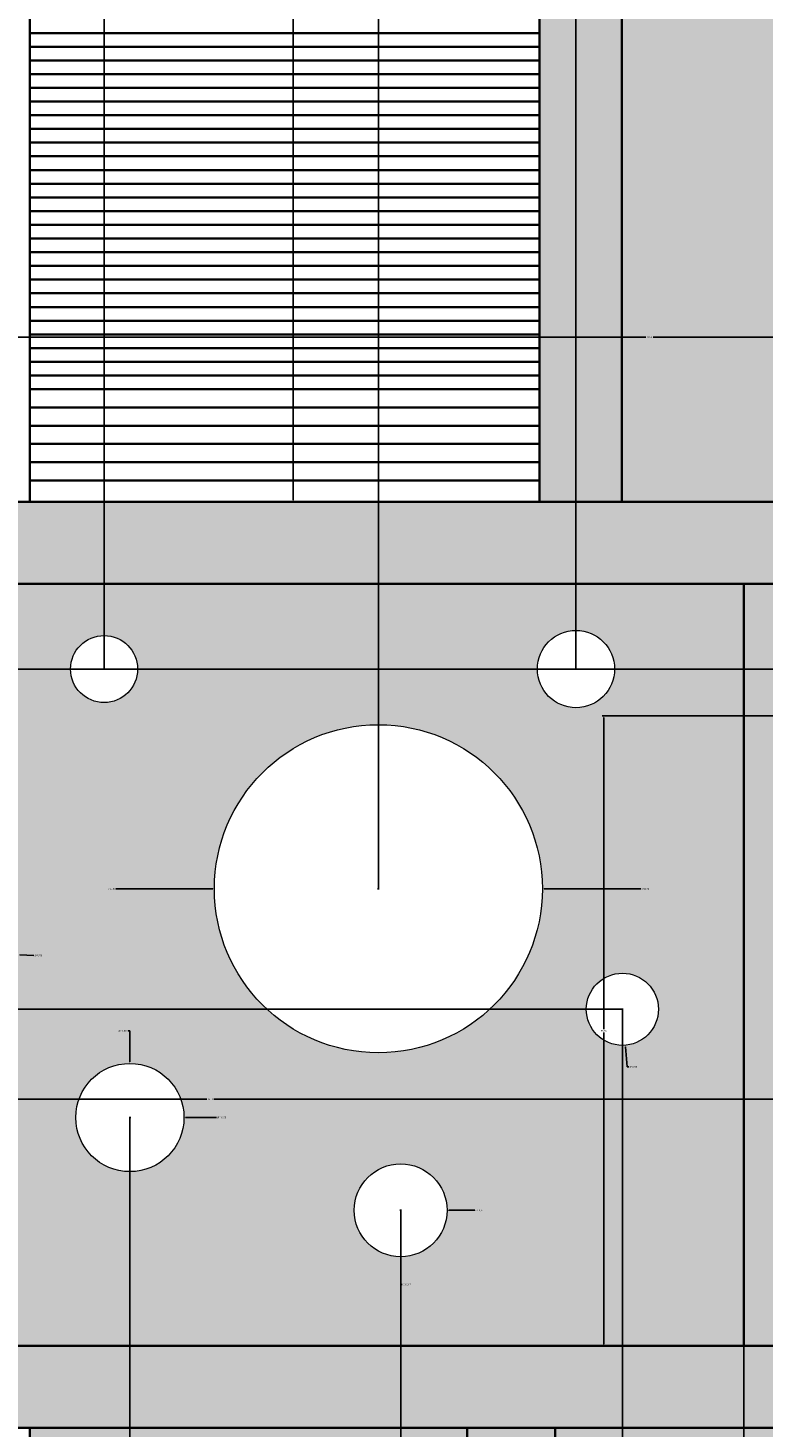
# Model space of a CAD drawing. Units: inches. Extents: x 73 to 607, y 92 to 651.
# Tile 14 of 18: x 256 to 337, y 311 to 465. Entities that reach past the tile are written whole.
import ezdxf

# ---------------------------------------------------------------- set-up
doc = ezdxf.new("R2010")
doc.units = ezdxf.units.IN
doc.header["$MEASUREMENT"] = 0
for name, color, linetype, lineweight in [('A-ANNO-DIMS', 2, 'Continuous', 18), ('A-ELEV', 7, 'Continuous', 35), ('A-ELEV-PANL', 7, 'Continuous', 18), ('A-ELEV-PATT-BKGD', 252, 'Continuous', 13), ('A-ELEV-PATT-SHAD', 8, 'Continuous', 13), ('A-ELEV-PATT-WALL', 254, 'Continuous', 13), ('A-ELEV-PATT-WOOD', 32, 'Continuous', 13)]:
    doc.layers.add(name, color=color, linetype=linetype, lineweight=lineweight)
doc.styles.get("Standard").update_dxf_attribs({"font": 'arial.ttf'})
doc.dimstyles.get("Standard").update_dxf_attribs({"dimtxt": 0.18, "dimasz": 0.18, "dimexe": 0.18, "dimexo": 0.0625, "dimgap": 0.09, "dimtad": 0, "dimtih": 1, "dimtoh": 1, "dimdec": 4, "dimzin": 0, "dimdsep": 46, "dimtxsty": 'Standard', "dimcen": 0.09, "dimadec": 0, "dimazin": 0, "dimtfac": 1, "dimtdec": 4, "dimtofl": 0, "dimtmove": 0, "dimatfit": 3, "dimfxl": 1, "dimtolj": 1, "dimtzin": 0, "dimarcsym": 0})

# ---------------------------------------------------------------- blocks, each defined once
blk = doc.blocks.new('*D5')
at = {"layer": 'A-ANNO-DIMS', "color": 0, "lineweight": -2, "transparency": 16777216}
for p, q in [((256.41, 623.8), (72.92, 623.8)), ((73.1, 623.62), (73.1, 383.68)), ((73.1, 143.38), (73.1, 383.32)), ((100.04, 143.2), (72.92, 143.2))]:
    blk.add_line(p, q, dxfattribs=at)
at = {"layer": 'A-ANNO-DIMS', "color": 0, "transparency": 16777216}
for points in [[(73.07, 623.62), (73.13, 623.62), (73.1, 623.8)], [(73.07, 143.38), (73.13, 143.38), (73.1, 143.2)]]:
    blk.add_solid(points, dxfattribs=at)
at = {"layer": 'Defpoints', "color": 0, "transparency": 16777216}
for p in [(73.1, 623.8), (256.47, 623.8), (100.1, 143.2)]:
    blk.add_point(p, dxfattribs=at)
at = {"layer": 'A-ANNO-DIMS', "color": 0, "transparency": 16777216, "insert": (73.1, 383.5), "char_height": 0.18, "attachment_point": 5}
blk.add_mtext('\\A1;480.6', dxfattribs=at)
blk = doc.blocks.new('*D44')
at = {"layer": 'A-ANNO-DIMS', "color": 0, "lineweight": -2, "transparency": 16777216}
for p, q in [((312.24, 543.16), (285.12, 543.16)), ((285.3, 542.98), (285.3, 478.08)), ((285.3, 412.82), (285.3, 477.71)), ((312.24, 412.64), (285.12, 412.64))]:
    blk.add_line(p, q, dxfattribs=at)
at = {"layer": 'A-ANNO-DIMS', "color": 0, "transparency": 16777216}
for points in [[(285.27, 542.98), (285.33, 542.98), (285.3, 543.16)], [(285.27, 412.82), (285.33, 412.82), (285.3, 412.64)]]:
    blk.add_solid(points, dxfattribs=at)
at = {"layer": 'Defpoints', "color": 0, "transparency": 16777216}
for p in [(285.3, 543.16), (312.3, 543.16), (312.3, 412.64)]:
    blk.add_point(p, dxfattribs=at)
at = {"layer": 'A-ANNO-DIMS', "color": 0, "transparency": 16777216, "insert": (285.3, 477.9), "char_height": 0.18, "attachment_point": 5}
blk.add_mtext('\\A1;130.52', dxfattribs=at)
blk = doc.blocks.new('*D45')
at = {"layer": 'A-ANNO-DIMS', "color": 0, "lineweight": -2, "transparency": 16777216}
for p, q in [((256.41, 552.16), (229.29, 552.16)), ((229.47, 551.98), (229.47, 482.58)), ((229.47, 412.82), (229.47, 482.21)), ((256.41, 412.64), (229.29, 412.64))]:
    blk.add_line(p, q, dxfattribs=at)
at = {"layer": 'A-ANNO-DIMS', "color": 0, "transparency": 16777216}
for points in [[(229.44, 551.98), (229.5, 551.98), (229.47, 552.16)], [(229.44, 412.82), (229.5, 412.82), (229.47, 412.64)]]:
    blk.add_solid(points, dxfattribs=at)
at = {"layer": 'Defpoints', "color": 0, "transparency": 16777216}
for p in [(229.47, 552.16), (256.47, 552.16), (256.47, 412.64)]:
    blk.add_point(p, dxfattribs=at)
at = {"layer": 'A-ANNO-DIMS', "color": 0, "transparency": 16777216, "insert": (229.47, 482.4), "char_height": 0.18, "attachment_point": 5}
blk.add_mtext('\\A1;139.52', dxfattribs=at)
blk = doc.blocks.new('*D52')
at = {"layer": 'A-ANNO-DIMS', "color": 0, "lineweight": -2, "transparency": 16777216}
for p, q in [((206.13, 403.7), (206.13, 430.82)), ((442.52, 403.7), (442.52, 430.82)), ((206.31, 430.64), (323.93, 430.64)), ((442.34, 430.64), (324.72, 430.64))]:
    blk.add_line(p, q, dxfattribs=at)
at = {"layer": 'A-ANNO-DIMS', "color": 0, "transparency": 16777216}
for points in [[(206.31, 430.67), (206.31, 430.61), (206.13, 430.64)], [(442.34, 430.67), (442.34, 430.61), (442.52, 430.64)]]:
    blk.add_solid(points, dxfattribs=at)
at = {"layer": 'Defpoints', "color": 0, "transparency": 16777216}
for p in [(442.52, 430.64), (206.13, 403.64), (442.52, 403.64)]:
    blk.add_point(p, dxfattribs=at)
at = {"layer": 'A-ANNO-DIMS', "color": 0, "transparency": 16777216, "insert": (324.33, 430.64), "char_height": 0.18, "attachment_point": 5}
blk.add_mtext('\\A1;236.4', dxfattribs=at)
blk = doc.blocks.new('*D54')
at = {"layer": 'A-ANNO-DIMS', "color": 0, "lineweight": -2, "transparency": 16777216}
for p, q in [((206.13, 320.27), (206.13, 347.38)), ((206.31, 347.2), (275.84, 347.2)), ((346.14, 347.2), (276.61, 347.2)), ((346.32, 320.27), (346.32, 347.38))]:
    blk.add_line(p, q, dxfattribs=at)
at = {"layer": 'A-ANNO-DIMS', "color": 0, "transparency": 16777216}
for points in [[(206.31, 347.23), (206.31, 347.17), (206.13, 347.2)], [(346.14, 347.23), (346.14, 347.17), (346.32, 347.2)]]:
    blk.add_solid(points, dxfattribs=at)
at = {"layer": 'Defpoints', "color": 0, "transparency": 16777216}
for p in [(346.32, 347.2), (206.13, 320.2), (346.32, 320.2)]:
    blk.add_point(p, dxfattribs=at)
at = {"layer": 'A-ANNO-DIMS', "color": 0, "transparency": 16777216, "insert": (276.23, 347.2), "char_height": 0.18, "attachment_point": 5}
blk.add_mtext('\\A1;140.2', dxfattribs=at)
blk = doc.blocks.new('*D56')
at = {"layer": 'A-ANNO-DIMS', "color": 0, "lineweight": -2, "transparency": 16777216}
for p, q in [((346.26, 389.18), (319.14, 389.18)), ((319.32, 389), (319.32, 354.87)), ((319.32, 320.38), (319.32, 354.51)), ((346.26, 320.2), (319.14, 320.2))]:
    blk.add_line(p, q, dxfattribs=at)
at = {"layer": 'A-ANNO-DIMS', "color": 0, "transparency": 16777216}
for points in [[(319.29, 389), (319.35, 389), (319.32, 389.18)], [(319.29, 320.38), (319.35, 320.38), (319.32, 320.2)]]:
    blk.add_solid(points, dxfattribs=at)
at = {"layer": 'Defpoints', "color": 0, "transparency": 16777216}
for p in [(319.32, 389.18), (346.32, 389.18), (346.32, 320.2)]:
    blk.add_point(p, dxfattribs=at)
at = {"layer": 'A-ANNO-DIMS', "color": 0, "transparency": 16777216, "insert": (319.32, 354.69), "char_height": 0.18, "attachment_point": 5}
blk.add_mtext('\\A1;68.98', dxfattribs=at)
blk = doc.blocks.new('*D59')
at = {"layer": 'A-ANNO-DIMS', "color": 0, "lineweight": -2, "transparency": 16777216}
for p, q in [((294.55, 370.25), (294.73, 370.25)), ((294.64, 370.16), (294.64, 370.34)), ((323.38, 370.25), (312.78, 370.25))]:
    blk.add_line(p, q, dxfattribs=at)
at = {"layer": 'A-ANNO-DIMS', "color": 0, "transparency": 16777216}
blk.add_solid([(312.78, 370.28), (312.78, 370.22), (312.6, 370.25)], dxfattribs=at)
at = {"layer": 'Defpoints', "color": 0, "transparency": 16777216}
for p in [(276.67, 370.25), (312.6, 370.25)]:
    blk.add_point(p, dxfattribs=at)
at = {"layer": 'A-ANNO-DIMS', "color": 0, "transparency": 16777216, "insert": (323.87, 370.25), "char_height": 0.18, "attachment_point": 5}
blk.add_mtext('\\A1;∅35.93', dxfattribs=at)
blk = doc.blocks.new('*D65')
at = {"layer": 'A-ANNO-DIMS', "color": 0, "lineweight": -2, "transparency": 16777216}
for p, q in [((267.33, 345.2), (267.51, 345.2)), ((267.42, 345.11), (267.42, 345.29)), ((276.9, 345.2), (273.52, 345.2))]:
    blk.add_line(p, q, dxfattribs=at)
at = {"layer": 'A-ANNO-DIMS', "color": 0, "transparency": 16777216}
blk.add_solid([(273.52, 345.23), (273.52, 345.17), (273.34, 345.2)], dxfattribs=at)
at = {"layer": 'Defpoints', "color": 0, "transparency": 16777216}
for p in [(261.49, 345.2), (273.34, 345.2)]:
    blk.add_point(p, dxfattribs=at)
at = {"layer": 'A-ANNO-DIMS', "color": 0, "transparency": 16777216, "insert": (277.46, 345.2), "char_height": 0.18, "attachment_point": 5}
blk.add_mtext('\\A1;∅11.855', dxfattribs=at)
blk = doc.blocks.new('*D67')
at = {"layer": 'A-ANNO-DIMS', "color": 0, "lineweight": -2, "transparency": 16777216}
for p, q in [((296.99, 335.04), (297.17, 335.04)), ((297.08, 334.95), (297.08, 335.13)), ((305.21, 335.04), (302.34, 335.04))]:
    blk.add_line(p, q, dxfattribs=at)
at = {"layer": 'A-ANNO-DIMS', "color": 0, "transparency": 16777216}
blk.add_solid([(302.34, 335.07), (302.34, 335.01), (302.16, 335.04)], dxfattribs=at)
at = {"layer": 'Defpoints', "color": 0, "transparency": 16777216}
for p in [(291.99, 335.04), (302.16, 335.04)]:
    blk.add_point(p, dxfattribs=at)
at = {"layer": 'A-ANNO-DIMS', "color": 0, "transparency": 16777216, "insert": (305.7, 335.04), "char_height": 0.18, "attachment_point": 5}
blk.add_mtext('\\A1;∅10.17', dxfattribs=at)
blk = doc.blocks.new('*D70')
at = {"layer": 'A-ANNO-DIMS', "color": 0, "lineweight": -2, "transparency": 16777216}
for p, q in [((241.43, 385.91), (241.43, 650.98)), ((241.61, 650.8), (252.54, 650.8)), ((264.41, 650.8), (253.47, 650.8)), ((264.59, 394.38), (264.59, 650.98))]:
    blk.add_line(p, q, dxfattribs=at)
at = {"layer": 'A-ANNO-DIMS', "color": 0, "transparency": 16777216}
for points in [[(241.61, 650.83), (241.61, 650.77), (241.43, 650.8)], [(264.41, 650.83), (264.41, 650.77), (264.59, 650.8)]]:
    blk.add_solid(points, dxfattribs=at)
at = {"layer": 'Defpoints', "color": 0, "transparency": 16777216}
for p in [(264.59, 650.8), (264.59, 394.31), (241.43, 385.85)]:
    blk.add_point(p, dxfattribs=at)
at = {"layer": 'A-ANNO-DIMS', "color": 0, "transparency": 16777216, "insert": (253.01, 650.8), "char_height": 0.18, "attachment_point": 5}
blk.add_mtext('\\A1;23.163', dxfattribs=at)
blk = doc.blocks.new('*D71')
at = {"layer": 'A-ANNO-DIMS', "color": 0, "lineweight": -2, "transparency": 16777216}
for p, q in [((264.59, 394.38), (264.59, 650.98)), ((264.77, 650.8), (279.15, 650.8)), ((294.46, 650.8), (280.08, 650.8)), ((294.64, 370.32), (294.64, 650.98))]:
    blk.add_line(p, q, dxfattribs=at)
at = {"layer": 'A-ANNO-DIMS', "color": 0, "transparency": 16777216}
for points in [[(264.77, 650.83), (264.77, 650.77), (264.59, 650.8)], [(294.46, 650.83), (294.46, 650.77), (294.64, 650.8)]]:
    blk.add_solid(points, dxfattribs=at)
at = {"layer": 'Defpoints', "color": 0, "transparency": 16777216}
for p in [(294.64, 650.8), (264.59, 394.31), (294.64, 370.25)]:
    blk.add_point(p, dxfattribs=at)
at = {"layer": 'A-ANNO-DIMS', "color": 0, "transparency": 16777216, "insert": (279.61, 650.8), "char_height": 0.18, "attachment_point": 5}
blk.add_mtext('\\A1;30.045', dxfattribs=at)
blk = doc.blocks.new('*D72')
at = {"layer": 'A-ANNO-DIMS', "color": 0, "lineweight": -2, "transparency": 16777216}
for p, q in [((294.64, 370.32), (294.64, 650.98)), ((294.82, 650.8), (305.06, 650.8)), ((316.1, 650.8), (305.86, 650.8)), ((316.28, 394.38), (316.28, 650.98))]:
    blk.add_line(p, q, dxfattribs=at)
at = {"layer": 'A-ANNO-DIMS', "color": 0, "transparency": 16777216}
for points in [[(294.82, 650.83), (294.82, 650.77), (294.64, 650.8)], [(316.1, 650.83), (316.1, 650.77), (316.28, 650.8)]]:
    blk.add_solid(points, dxfattribs=at)
at = {"layer": 'Defpoints', "color": 0, "transparency": 16777216}
for p in [(316.28, 650.8), (316.28, 394.31), (294.64, 370.25)]:
    blk.add_point(p, dxfattribs=at)
at = {"layer": 'A-ANNO-DIMS', "color": 0, "transparency": 16777216, "insert": (305.46, 650.8), "char_height": 0.18, "attachment_point": 5}
blk.add_mtext('\\A1;21.65', dxfattribs=at)
blk = doc.blocks.new('*D75')
at = {"layer": 'A-ANNO-DIMS', "color": 0, "lineweight": -2, "transparency": 16777216}
for p, q in [((252.34, 363.04), (252.34, 116.02)), ((267.42, 345.14), (267.42, 116.02)), ((252.52, 116.2), (259.42, 116.2)), ((267.24, 116.2), (260.33, 116.2))]:
    blk.add_line(p, q, dxfattribs=at)
at = {"layer": 'A-ANNO-DIMS', "color": 0, "transparency": 16777216}
for points in [[(252.52, 116.23), (252.52, 116.17), (252.34, 116.2)], [(267.24, 116.23), (267.24, 116.17), (267.42, 116.2)]]:
    blk.add_solid(points, dxfattribs=at)
at = {"layer": 'Defpoints', "color": 0, "transparency": 16777216}
for p in [(252.34, 363.11), (267.42, 345.2), (267.42, 116.2)]:
    blk.add_point(p, dxfattribs=at)
at = {"layer": 'A-ANNO-DIMS', "color": 0, "transparency": 16777216, "insert": (259.88, 116.2), "char_height": 0.18, "attachment_point": 5}
blk.add_mtext('\\A1;15.074', dxfattribs=at)
blk = doc.blocks.new('*D76')
at = {"layer": 'A-ANNO-DIMS', "color": 0, "lineweight": -2, "transparency": 16777216}
for p, q in [((267.42, 345.14), (267.42, 116.02)), ((297.08, 334.98), (297.08, 116.02)), ((267.6, 116.2), (281.85, 116.2)), ((296.9, 116.2), (282.64, 116.2))]:
    blk.add_line(p, q, dxfattribs=at)
at = {"layer": 'A-ANNO-DIMS', "color": 0, "transparency": 16777216}
for points in [[(267.6, 116.23), (267.6, 116.17), (267.42, 116.2)], [(296.9, 116.23), (296.9, 116.17), (297.08, 116.2)]]:
    blk.add_solid(points, dxfattribs=at)
at = {"layer": 'Defpoints', "color": 0, "transparency": 16777216}
for p in [(267.42, 345.2), (297.08, 335.04), (297.08, 116.2)]:
    blk.add_point(p, dxfattribs=at)
at = {"layer": 'A-ANNO-DIMS', "color": 0, "transparency": 16777216, "insert": (282.25, 116.2), "char_height": 0.18, "attachment_point": 5}
blk.add_mtext('\\A1;29.66', dxfattribs=at)
blk = doc.blocks.new('*D77')
at = {"layer": 'A-ANNO-DIMS', "color": 0, "lineweight": -2, "transparency": 16777216}
for p, q in [((321.37, 356.99), (321.37, 116.02)), ((334.67, 320.14), (334.67, 116.02)), ((321.55, 116.2), (327.63, 116.2)), ((334.49, 116.2), (328.4, 116.2))]:
    blk.add_line(p, q, dxfattribs=at)
at = {"layer": 'A-ANNO-DIMS', "color": 0, "transparency": 16777216}
for points in [[(321.55, 116.23), (321.55, 116.17), (321.37, 116.2)], [(334.49, 116.23), (334.49, 116.17), (334.67, 116.2)]]:
    blk.add_solid(points, dxfattribs=at)
at = {"layer": 'Defpoints', "color": 0, "transparency": 16777216}
for p in [(321.37, 357.06), (334.67, 320.2), (321.37, 116.2)]:
    blk.add_point(p, dxfattribs=at)
at = {"layer": 'A-ANNO-DIMS', "color": 0, "transparency": 16777216, "insert": (328.02, 116.2), "char_height": 0.18, "attachment_point": 5}
blk.add_mtext('\\A1;13.30', dxfattribs=at)
blk = doc.blocks.new('*D79')
at = {"layer": 'A-ANNO-DIMS', "color": 0, "lineweight": -2, "transparency": 16777216}
for p, q in [((334.73, 403.64), (607.28, 403.64)), ((607.1, 403.46), (607.1, 399.16)), ((607.1, 394.49), (607.1, 398.79)), ((316.35, 394.31), (607.28, 394.31))]:
    blk.add_line(p, q, dxfattribs=at)
at = {"layer": 'A-ANNO-DIMS', "color": 0, "transparency": 16777216}
for points in [[(607.07, 403.46), (607.13, 403.46), (607.1, 403.64)], [(607.07, 394.49), (607.13, 394.49), (607.1, 394.31)]]:
    blk.add_solid(points, dxfattribs=at)
at = {"layer": 'Defpoints', "color": 0, "transparency": 16777216}
for p in [(334.67, 403.64), (316.28, 394.31), (607.1, 394.31)]:
    blk.add_point(p, dxfattribs=at)
at = {"layer": 'A-ANNO-DIMS', "color": 0, "transparency": 16777216, "insert": (607.1, 398.98), "char_height": 0.18, "attachment_point": 5}
blk.add_mtext('\\A1;9.322', dxfattribs=at)
blk = doc.blocks.new('*D80')
at = {"layer": 'A-ANNO-DIMS', "color": 0, "lineweight": -2, "transparency": 16777216}
for p, q in [((316.22, 394.31), (72.92, 394.31)), ((73.1, 394.13), (73.1, 375.87)), ((73.1, 357.24), (73.1, 375.5)), ((321.31, 357.06), (72.92, 357.06))]:
    blk.add_line(p, q, dxfattribs=at)
at = {"layer": 'A-ANNO-DIMS', "color": 0, "transparency": 16777216}
for points in [[(73.07, 394.13), (73.13, 394.13), (73.1, 394.31)], [(73.07, 357.24), (73.13, 357.24), (73.1, 357.06)]]:
    blk.add_solid(points, dxfattribs=at)
at = {"layer": 'Defpoints', "color": 0, "transparency": 16777216}
for p in [(316.28, 394.31), (73.1, 357.06), (321.37, 357.06)]:
    blk.add_point(p, dxfattribs=at)
at = {"layer": 'A-ANNO-DIMS', "color": 0, "transparency": 16777216, "insert": (73.1, 375.69), "char_height": 0.18, "attachment_point": 5}
blk.add_mtext('\\A1;37.26', dxfattribs=at)
blk = doc.blocks.new('*D134')
at = {"layer": 'A-ANNO-DIMS', "color": 0, "lineweight": -2, "transparency": 16777216}
for p, q in [((264.5, 394.31), (264.68, 394.31)), ((264.59, 394.22), (264.59, 394.4)), ((270.46, 394.29), (268.44, 394.3))]:
    blk.add_line(p, q, dxfattribs=at)
at = {"layer": 'A-ANNO-DIMS', "color": 0, "transparency": 16777216}
blk.add_solid([(268.44, 394.33), (268.44, 394.27), (268.26, 394.3)], dxfattribs=at)
at = {"layer": 'Defpoints', "color": 0, "transparency": 16777216}
for p in [(260.92, 394.33), (268.26, 394.3)]:
    blk.add_point(p, dxfattribs=at)
at = {"layer": 'A-ANNO-DIMS', "color": 0, "transparency": 16777216, "insert": (270.95, 394.29), "char_height": 0.18, "attachment_point": 5}
blk.add_mtext('\\A1;∅7.339', dxfattribs=at)
blk = doc.blocks.new('*D135')
at = {"layer": 'A-ANNO-DIMS', "color": 0, "lineweight": -2, "transparency": 16777216}
for p, q in [((316.19, 394.31), (316.37, 394.31)), ((316.28, 394.22), (316.28, 394.4)), ((323.06, 394.29), (320.7, 394.3))]:
    blk.add_line(p, q, dxfattribs=at)
at = {"layer": 'A-ANNO-DIMS', "color": 0, "transparency": 16777216}
blk.add_solid([(320.7, 394.33), (320.7, 394.27), (320.52, 394.3)], dxfattribs=at)
at = {"layer": 'Defpoints', "color": 0, "transparency": 16777216}
for p in [(312.05, 394.33), (320.52, 394.3)]:
    blk.add_point(p, dxfattribs=at)
at = {"layer": 'A-ANNO-DIMS', "color": 0, "transparency": 16777216, "insert": (323.55, 394.29), "char_height": 0.18, "attachment_point": 5}
blk.add_mtext('\\A1;∅8.468', dxfattribs=at)
blk = doc.blocks.new('*D136')
at = {"layer": 'A-ANNO-DIMS', "color": 0, "lineweight": -2, "transparency": 16777216}
for p, q in [((265.89, 370.25), (276.49, 370.25)), ((294.55, 370.25), (294.73, 370.25)), ((294.64, 370.16), (294.64, 370.34))]:
    blk.add_line(p, q, dxfattribs=at)
at = {"layer": 'A-ANNO-DIMS', "color": 0, "transparency": 16777216}
blk.add_solid([(276.49, 370.28), (276.49, 370.22), (276.67, 370.25)], dxfattribs=at)
at = {"layer": 'Defpoints', "color": 0, "transparency": 16777216}
for p in [(276.67, 370.25), (312.6, 370.26)]:
    blk.add_point(p, dxfattribs=at)
at = {"layer": 'A-ANNO-DIMS', "color": 0, "transparency": 16777216, "insert": (265.4, 370.25), "char_height": 0.18, "attachment_point": 5}
blk.add_mtext('\\A1;∅35.93', dxfattribs=at)
blk = doc.blocks.new('*D137')
at = {"layer": 'A-ANNO-DIMS', "color": 0, "lineweight": -2, "transparency": 16777216}
for p, q in [((252.25, 363.11), (252.43, 363.11)), ((252.34, 363.02), (252.34, 363.2)), ((256.88, 362.94), (255.36, 363))]:
    blk.add_line(p, q, dxfattribs=at)
at = {"layer": 'A-ANNO-DIMS', "color": 0, "transparency": 16777216}
blk.add_solid([(255.36, 363.03), (255.36, 362.97), (255.18, 363)], dxfattribs=at)
at = {"layer": 'Defpoints', "color": 0, "transparency": 16777216}
for p in [(249.5, 363.21), (255.18, 363)]:
    blk.add_point(p, dxfattribs=at)
at = {"layer": 'A-ANNO-DIMS', "color": 0, "transparency": 16777216, "insert": (257.37, 362.94), "char_height": 0.18, "attachment_point": 5}
blk.add_mtext('\\A1;∅5.679', dxfattribs=at)
blk = doc.blocks.new('*D138')
at = {"layer": 'A-ANNO-DIMS', "color": 0, "lineweight": -2, "transparency": 16777216}
for p, q in [((321.28, 357.06), (321.46, 357.06)), ((321.37, 356.97), (321.37, 357.15)), ((321.89, 350.76), (321.71, 352.94)), ((322.07, 350.76), (321.89, 350.76))]:
    blk.add_line(p, q, dxfattribs=at)
at = {"layer": 'A-ANNO-DIMS', "color": 0, "transparency": 16777216}
blk.add_solid([(321.74, 352.94), (321.68, 352.94), (321.69, 353.12)], dxfattribs=at)
at = {"layer": 'Defpoints', "color": 0, "transparency": 16777216}
for p in [(321.04, 361), (321.69, 353.12)]:
    blk.add_point(p, dxfattribs=at)
at = {"layer": 'A-ANNO-DIMS', "color": 0, "transparency": 16777216, "insert": (322.56, 350.76), "char_height": 0.18, "attachment_point": 5}
blk.add_mtext('\\A1;∅7.903', dxfattribs=at)
blk = doc.blocks.new('*D140')
at = {"layer": 'A-ANNO-DIMS', "color": 0, "lineweight": -2, "transparency": 16777216}
for p, q in [((267.23, 354.69), (267.41, 354.69)), ((267.41, 354.69), (267.41, 351.31)), ((267.33, 345.2), (267.51, 345.2)), ((267.42, 345.11), (267.42, 345.29))]:
    blk.add_line(p, q, dxfattribs=at)
at = {"layer": 'A-ANNO-DIMS', "color": 0, "transparency": 16777216}
blk.add_solid([(267.44, 351.31), (267.38, 351.31), (267.41, 351.13)], dxfattribs=at)
at = {"layer": 'Defpoints', "color": 0, "transparency": 16777216}
for p in [(267.41, 351.13), (267.42, 339.28)]:
    blk.add_point(p, dxfattribs=at)
at = {"layer": 'A-ANNO-DIMS', "color": 0, "transparency": 16777216, "insert": (266.66, 354.69), "char_height": 0.18, "attachment_point": 5}
blk.add_mtext('\\A1;∅11.855', dxfattribs=at)
blk = doc.blocks.new('*D141')
at = {"layer": 'A-ANNO-DIMS', "color": 0, "lineweight": -2, "transparency": 16777216}
for p, q in [((296.99, 335.04), (297.17, 335.04)), ((297.08, 334.95), (297.08, 335.13)), ((297.08, 326.91), (297.08, 329.78)), ((297.26, 326.91), (297.08, 326.91))]:
    blk.add_line(p, q, dxfattribs=at)
at = {"layer": 'A-ANNO-DIMS', "color": 0, "transparency": 16777216}
blk.add_solid([(297.11, 329.78), (297.05, 329.78), (297.08, 329.96)], dxfattribs=at)
at = {"layer": 'Defpoints', "color": 0, "transparency": 16777216}
for p in [(297.07, 340.13), (297.08, 329.96)]:
    blk.add_point(p, dxfattribs=at)
at = {"layer": 'A-ANNO-DIMS', "color": 0, "transparency": 16777216, "insert": (297.75, 326.91), "char_height": 0.18, "attachment_point": 5}
blk.add_mtext('\\A1;∅10.17', dxfattribs=at)

msp = doc.modelspace()

# ---------------------------------------------------------------- hatches: boundary and pattern name
at = {"layer": 'A-ELEV-PATT-BKGD'}
h = msp.add_hatch(color=256, dxfattribs=at)
h.dxf.hatch_style = 1
h.paths.add_polyline_path([(321.3008, 479.2042), (312.3008, 479.2042), (312.3008, 478.7576), (312.3008, 412.636), (321.3008, 412.636)])
h.paths.add_polyline_path([(312.3008, 504.7576), (256.4726, 504.7576), (256.4726, 503.4576), (312.3008, 503.4576)], flags=17)
h.paths.add_polyline_path([(321.3008, 543.1576), (321.3008, 552.1576), (320.3257, 552.1576), (312.3008, 552.1576), (256.4726, 552.1576), (256.4726, 543.1576), (312.3008, 543.1576), (312.3008, 479.2042), (321.3008, 479.2042)])
h.paths.add_polyline_path([(451.5214, 412.636), (256.4726, 412.636), (256.4726, 403.636), (442.5214, 403.636), (442.5214, 320.2042), (206.1343, 320.2042), (206.1343, 320.9135), (206.1343, 403.636), (256.4726, 403.636), (256.4726, 412.636), (201.6343, 412.636), (201.6343, 320.9135), (201.6343, 320.2042), (201.6343, 311.2042), (256.4726, 311.2042), (451.5214, 311.2042)])
h.paths.add_polyline_path([(431.07, 258.6914), (369.5339, 258.6914), (369.5339, 247.4054), (396.692, 247.4054), (425.07, 247.4054), (425.07, 194.7312), (396.692, 194.6197), (396.692, 194.5366), (369.5339, 194.5366), (369.5339, 185.6619), (431.07, 185.6619)])
h.paths.add_polyline_path([(580.0983, 262.3024), (451.5214, 262.3024), (451.5214, 143.2042), (580.0983, 143.2042)])
h.paths.add_polyline_path([(454.7049, 174.802), (454.7049, 256.6321), (577.9249, 256.6321), (577.9249, 174.802)], flags=16)
h.paths.add_polyline_path([(465.9716, 191.1416, -1), (473.7874, 191.1416, -1)], flags=0)
h.paths.add_polyline_path([(490.5373, 181.6586, -1), (494.9999, 181.6586, -1)], flags=0)
h.paths.add_polyline_path([(476.2996, 209.8287, -1), (500.5844, 209.8287, -1)], flags=0)
h.paths.add_polyline_path([(505.3326, 194.7675, -1), (512.5843, 194.7675, -1)], flags=0)
h.paths.add_polyline_path([(520.9613, 186.679, -1), (526.544, 186.679, -1)], flags=0)
h.paths.add_polyline_path([(466.8103, 225.7267, -1), (470.1573, 225.7267, -1)], flags=0)
h.paths.add_polyline_path([(527.1059, 203.6926, -1), (536.0311, 203.6926, -1)], flags=0)
h.paths.add_polyline_path([(504.775, 232.6995, -1), (513.7002, 232.6995, -1)], flags=0)
h.paths.add_polyline_path([(546.9241, 183.611, -1), (554.7336, 183.611, -1)], flags=0)
h.paths.add_polyline_path([(459.5544, 243.856, -1), (466.8061, 243.856, -1)], flags=0)
h.paths.add_polyline_path([(476.3045, 246.924, -1), (488.5767, 246.924, -1)], flags=0)
h.paths.add_polyline_path([(529.9044, 226.8424, -1), (556.68, 226.8424, -1)], flags=0)
h.paths.add_polyline_path([(554.1814, 203.9716, -1), (561.4331, 203.9716, -1)], flags=0)
h.paths.add_polyline_path([(567.8561, 193.3729, -1), (570.6475, 193.3729, -1)], flags=0)
h.paths.add_polyline_path([(522.3584, 250.271, -1), (525.7053, 250.271, -1)], flags=0)
h.paths.add_polyline_path([(561.9965, 245.2506, -1), (567.5748, 245.2506, -1)], flags=0)
h.paths.add_polyline_path([(347.8686, 194.5366), (341.8686, 194.5366), (341.8686, 194.5452), (314.0144, 194.5452), (314.0144, 188.5452), (347.8686, 188.5452)])
h.paths.add_polyline_path([(347.8686, 253.4054), (314.0144, 253.4054), (314.0144, 247.4054), (341.8686, 247.4054), (347.8686, 247.4054)])
h.paths.add_polyline_path([(304.3559, 253.4054), (298.3559, 253.4054), (298.3559, 188.5452), (304.3559, 188.5452)])
h.paths.add_polyline_path([(450.6603, 552.1576), (369.9727, 552.1576), (369.9727, 479.2042), (374.4727, 479.2042), (374.4727, 547.6576), (446.1603, 547.6576), (446.1603, 479.2042), (450.6603, 479.2042)])
h.paths.add_polyline_path([(374.4727, 479.2042), (369.9727, 479.2042), (369.9727, 465.0632), (374.4727, 465.0632)])
h.paths.add_polyline_path([(450.6603, 479.2042), (446.1603, 479.2042), (446.1603, 465.0632), (450.6603, 465.0632)])
h.paths.add_polyline_path([(256.4726, 281.6039), (109.0983, 281.6039), (100.0983, 281.6039), (100.0983, 167.2042), (100.0983, 143.2042), (109.0983, 143.2042), (109.0983, 167.2042), (109.0983, 272.6039), (256.4726, 272.6039)])
at = {"layer": 'A-ELEV-PATT-SHAD'}
h = msp.add_hatch(color=256, dxfattribs=at)
h.dxf.hatch_style = 1
h.paths.add_polyline_path([(451.5214, 412.636), (256.4726, 412.636), (256.4726, 403.636), (442.5214, 403.636), (442.5214, 320.2042), (206.1343, 320.2042), (206.1343, 320.9135), (206.1343, 403.636), (256.4726, 403.636), (256.4726, 412.636), (201.6343, 412.636), (201.6343, 320.9135), (201.6343, 320.2042), (201.6343, 311.2042), (256.4726, 311.2042), (451.5214, 311.2042)])
h.paths.add_polyline_path([(580.0983, 262.3024), (451.5214, 262.3024), (451.5214, 143.2042), (580.0983, 143.2042)])
h.paths.add_polyline_path([(454.7049, 174.802), (454.7049, 256.6321), (577.9249, 256.6321), (577.9249, 174.802)], flags=16)
h.paths.add_polyline_path([(465.9716, 191.1416, -1), (473.7874, 191.1416, -1)], flags=0)
h.paths.add_polyline_path([(490.5373, 181.6586, -1), (494.9999, 181.6586, -1)], flags=0)
h.paths.add_polyline_path([(476.2996, 209.8287, -1), (500.5844, 209.8287, -1)], flags=0)
h.paths.add_polyline_path([(505.3326, 194.7675, -1), (512.5843, 194.7675, -1)], flags=0)
h.paths.add_polyline_path([(520.9613, 186.679, -1), (526.544, 186.679, -1)], flags=0)
h.paths.add_polyline_path([(466.8103, 225.7267, -1), (470.1573, 225.7267, -1)], flags=0)
h.paths.add_polyline_path([(527.1059, 203.6926, -1), (536.0311, 203.6926, -1)], flags=0)
h.paths.add_polyline_path([(459.5544, 243.856, -1), (466.8061, 243.856, -1)], flags=0)
h.paths.add_polyline_path([(504.775, 232.6995, -1), (513.7002, 232.6995, -1)], flags=0)
h.paths.add_polyline_path([(476.3045, 246.924, -1), (488.5767, 246.924, -1)], flags=0)
h.paths.add_polyline_path([(546.9241, 183.611, -1), (554.7336, 183.611, -1)], flags=0)
h.paths.add_polyline_path([(529.9044, 226.8424, -1), (556.68, 226.8424, -1)], flags=0)
h.paths.add_polyline_path([(554.1814, 203.9716, -1), (561.4331, 203.9716, -1)], flags=0)
h.paths.add_polyline_path([(522.3584, 250.271, -1), (525.7053, 250.271, -1)], flags=0)
h.paths.add_polyline_path([(567.8561, 193.3729, -1), (570.6475, 193.3729, -1)], flags=0)
h.paths.add_polyline_path([(561.9965, 245.2506, -1), (567.5748, 245.2506, -1)], flags=0)
h.paths.add_polyline_path([(431.07, 258.6914), (369.5339, 258.6914), (369.5339, 247.4054), (396.692, 247.4054), (425.07, 247.4054), (425.07, 194.7312), (396.692, 194.6197), (396.692, 194.5366), (369.5339, 194.5366), (369.5339, 185.6619), (431.07, 185.6619)])
h.paths.add_polyline_path([(347.8686, 253.4054), (314.0144, 253.4054), (314.0144, 247.4054), (341.8686, 247.4054), (347.8686, 247.4054)])
h.paths.add_polyline_path([(304.3559, 253.4054), (298.3559, 253.4054), (298.3559, 188.5452), (304.3559, 188.5452)])
h.paths.add_polyline_path([(347.8686, 194.5366), (341.8686, 194.5366), (341.8686, 194.5452), (314.0144, 194.5452), (314.0144, 188.5452), (347.8686, 188.5452)])
h = msp.add_hatch(color=256, dxfattribs=at)
h.dxf.hatch_style = 1
h.paths.add_polyline_path([(338.6695, 403.636), (334.6695, 403.636), (334.6695, 320.2042), (338.6695, 320.2042)])
at = {"layer": 'A-ELEV-PATT-WALL'}
h = msp.add_hatch(color=256, dxfattribs=at)
h.dxf.hatch_style = 1
h.paths.add_polyline_path([(509.9692, 483.857), (450.6603, 483.857), (450.6603, 465.0632), (446.1603, 465.0632), (446.1603, 484.2142), (374.4727, 484.2142), (374.4727, 465.0632), (369.9727, 465.0632), (369.9727, 484.2142), (321.3008, 484.2142), (321.3008, 412.636), (451.5214, 412.636), (451.5214, 311.2042), (314.0144, 311.2042), (314.0144, 253.4054), (347.8686, 253.4054), (347.8686, 247.4054), (369.5339, 247.4054), (369.5339, 258.6914), (431.07, 258.6914), (431.07, 185.6619), (369.5339, 185.6619), (369.5339, 194.5366), (347.8686, 194.5366), (347.8686, 188.5452), (314.0144, 188.5452), (314.0144, 143.2042), (451.5214, 143.2042), (451.5214, 262.3024), (580.0983, 262.3024), (580.0983, 311.2042), (509.9692, 311.2042)])
h.paths.add_polyline_path([(304.3559, 311.2042), (256.4726, 311.2042), (256.4726, 167.2042), (256.4726, 143.2042), (304.3559, 143.2042), (304.3559, 188.5452), (298.3559, 188.5452), (298.3559, 253.4054), (304.3559, 253.4054)])
at = {"layer": 'A-ELEV-PATT-WOOD'}
h = msp.add_hatch(color=256, dxfattribs=at)
h.dxf.hatch_style = 1
h.paths.add_polyline_path([(256.4726, 403.636), (206.1343, 403.636), (206.1343, 320.9135), (206.1343, 320.2042), (256.4726, 320.2042)])
h.paths.add_polyline_path([(217.9817, 392.9028, -1), (226.456, 392.9028, -1)], flags=16)
h.paths.add_polyline_path([(232.9598, 385.8466, -1), (249.8948, 385.8466, -1)], flags=16)
h.paths.add_polyline_path([(240.6496, 347.1939, -1), (210.9085, 347.1939, -1)], flags=16)
h.paths.add_polyline_path([(255.1802, 363.1072, -1), (249.5015, 363.1072, -1)], flags=16)
h.paths.add_polyline_path([(334.6695, 403.636), (256.4726, 403.636), (256.4726, 320.2042), (334.6695, 320.2042)])
h.paths.add_polyline_path([(312.5994, 370.2541, -1), (276.6709, 370.2541, -1)], flags=16)
h.paths.add_polyline_path([(260.9211, 394.3141, -1), (268.2596, 394.3141, -1)], flags=16)
h.paths.add_polyline_path([(273.3424, 345.2025, -1), (261.4879, 345.2025, -1)], flags=16)
h.paths.add_polyline_path([(302.1597, 335.0415, -1), (291.9906, 335.0415, -1)], flags=16)
h.paths.add_polyline_path([(312.0498, 394.3141, -1), (320.5173, 394.3141, -1)], flags=16)
h.paths.add_polyline_path([(325.3197, 357.0571, -1), (317.4166, 357.0571, -1)], flags=16)
h = msp.add_hatch(color=256, dxfattribs=at)
h.dxf.hatch_style = 1
h.paths.add_polyline_path([(314.0144, 311.2042), (304.3559, 311.2042), (304.3559, 143.2042), (314.0144, 143.2042)])

# ---------------------------------------------------------------- linework, layer by layer
at = {"layer": 'A-ELEV'}
for p, q in [((312.3008, 412.636), (312.3008, 543.1576)), ((321.3008, 412.636), (321.3008, 543.1576)), ((256.4726, 455.2042), (256.4726, 503.2042)), ((312.3008, 463.9576), (256.4726, 463.9576)), ((312.3008, 462.4576), (256.4726, 462.4576)), ((312.3008, 460.9576), (256.4726, 460.9576)), ((312.3008, 459.4576), (256.4726, 459.4576)), ((312.3008, 457.9576), (256.4726, 457.9576)), ((312.3008, 456.4576), (256.4726, 456.4576)), ((256.4726, 456.4576), (256.4726, 412.636)), ((312.3008, 454.9576), (256.4726, 454.9576)), ((312.3008, 453.4576), (256.4726, 453.4576)), ((312.3008, 451.9576), (256.4726, 451.9576)), ((312.3008, 450.4576), (256.4726, 450.4576)), ((312.3008, 448.9576), (256.4726, 448.9576)), ((312.3008, 447.4576), (256.4726, 447.4576)), ((312.3008, 445.9576), (256.4726, 445.9576)), ((312.3008, 444.4576), (256.4726, 444.4576)), ((312.3008, 442.9576), (256.4726, 442.9576)), ((312.3008, 441.4576), (256.4726, 441.4576)), ((312.3008, 439.9576), (256.4726, 439.9576)), ((312.3008, 438.4576), (256.4726, 438.4576)), ((312.3008, 436.9576), (256.4726, 436.9576)), ((312.3008, 435.4576), (256.4726, 435.4576)), ((312.3008, 433.9576), (256.4726, 433.9576)), ((312.3008, 432.4576), (256.4726, 432.4576)), ((312.3008, 430.9576), (256.4726, 430.9576)), ((312.3008, 429.4576), (256.4726, 429.4576)), ((312.3008, 427.9576), (256.4726, 427.9576)), ((312.3008, 426.4576), (256.4726, 426.4576)), ((312.3008, 424.9576), (256.4726, 424.9576)), ((312.3008, 422.9576), (256.4726, 422.9576)), ((312.3008, 420.9576), (256.4726, 420.9576)), ((312.3008, 418.9576), (256.4726, 418.9576)), ((312.3008, 416.9576), (256.4726, 416.9576)), ((312.3008, 414.9576), (256.4726, 414.9576)), ((451.5214, 412.636), (201.6343, 412.636)), ((442.5214, 403.636), (206.1343, 403.636)), ((334.6695, 320.2042), (334.6695, 403.636)), ((206.1343, 320.2042), (442.5214, 320.2042)), ((256.4726, 320.2042), (256.4726, 320.2042)), ((256.4726, 311.2042), (201.6343, 311.2042)), ((256.4726, 311.2042), (256.4726, 167.2042)), ((451.5214, 311.2042), (256.4726, 311.2042))]:
    msp.add_line(p, q, dxfattribs=at)
msp.add_lwpolyline([(304.3559, 143.2042), (314.0144, 143.2042), (314.0144, 311.2042), (304.3559, 311.2042)], close=True, dxfattribs=at)
at = {"layer": 'A-ELEV-PANL'}
for centre, radius in [((264.5904, 394.3141), 3.6693), ((316.2836, 394.3141), 4.2338), ((294.6352, 370.2541), 17.9643), ((321.3681, 357.0571), 3.9515), ((267.4151, 345.2025), 5.9273), ((297.0752, 335.0415), 5.0846)]:
    msp.add_circle(centre, radius, dxfattribs=at)

# ---------------------------------------------------------------- dimensions: what is measured, and where the dimension line sits
at = {"layer": 'A-ANNO-DIMS'}
for base, p1, p2, override, picture, middle in [((264.5904, 650.801), (241.4273, 385.8466), (264.5904, 394.3141), {"dimdec": 3, "dimlfac": 1, "dimrnd": 0, "dimzin": 0, "dimdsep": 46, "dimlunit": 2}, '*D70', (253.0088, 650.801)), ((294.6352, 650.801), (264.5904, 394.3141), (294.6352, 370.2541), {"dimdec": 3, "dimlfac": 1, "dimrnd": 0, "dimzin": 0, "dimdsep": 46, "dimlunit": 2}, '*D71', (279.6128, 650.801)), ((316.2836, 650.801), (294.6352, 370.2541), (316.2836, 394.3141), {"dimdec": 2, "dimlfac": 1, "dimrnd": 0, "dimzin": 0, "dimdsep": 46, "dimlunit": 2}, '*D72', (305.4594, 650.801)), ((442.5214, 430.636), (206.1343, 403.636), (442.5214, 403.636), {"dimdec": 1, "dimlfac": 1, "dimrnd": 0, "dimzin": 0, "dimdsep": 46, "dimlunit": 2}, '*D52', (324.3278, 430.636)), ((267.4151, 116.2042), (252.3408, 363.1072), (267.4151, 345.2025), {"dimdec": 3, "dimlfac": 1, "dimrnd": 0, "dimzin": 0, "dimdsep": 46, "dimlunit": 2}, '*D75', (259.878, 116.2042)), ((321.3681, 116.2042), (334.6695, 320.2042), (321.3681, 357.0571), {"dimdec": 2, "dimlfac": 1, "dimrnd": 0, "dimzin": 0, "dimdsep": 46, "dimlunit": 2}, '*D77', (328.0188, 116.2042)), ((346.3213, 347.2042), (206.1343, 320.2042), (346.3213, 320.2042), {"dimdec": 1, "dimlfac": 1, "dimrnd": 0, "dimzin": 0, "dimdsep": 46, "dimlunit": 2}, '*D54', (276.2278, 347.2042)), ((297.0752, 116.2042), (267.4151, 345.2025), (297.0752, 335.0415), {"dimdec": 2, "dimlfac": 1, "dimrnd": 0, "dimzin": 0, "dimdsep": 46, "dimlunit": 2}, '*D76', (282.2451, 116.2042))]:
    dim = msp.add_linear_dim(base=base, p1=p1, p2=p2, dimstyle='Standard', override=override, dxfattribs=at)
    dim.commit()
    dim.dimension.update_dxf_attribs({"geometry": picture, "text_midpoint": middle})
for base, p1, p2, override, picture, middle in [((73.0983, 623.801), (100.0983, 143.2042), (256.4726, 623.801), {"dimdec": 1, "dimlfac": 1, "dimrnd": 0, "dimzin": 0, "dimdsep": 46, "dimlunit": 2}, '*D5', (73.0983, 383.5026)), ((229.4726, 552.1576), (256.4726, 412.636), (256.4726, 552.1576), {"dimdec": 2, "dimlfac": 1, "dimrnd": 0, "dimzin": 0, "dimdsep": 46, "dimlunit": 2}, '*D45', (229.4726, 482.3968)), ((285.3008, 543.1576), (312.3008, 412.636), (312.3008, 543.1576), {"dimdec": 2, "dimlfac": 1, "dimrnd": 0, "dimzin": 0, "dimdsep": 46, "dimlunit": 2}, '*D44', (285.3008, 477.8968)), ((607.0983, 394.3141), (334.6695, 403.636), (316.2836, 394.3141), {"dimdec": 3, "dimlfac": 1, "dimrnd": 0, "dimzin": 0, "dimdsep": 46, "dimlunit": 2}, '*D79', (607.0983, 398.9751)), ((73.0983, 357.0571), (316.2836, 394.3141), (321.3681, 357.0571), {"dimdec": 2, "dimlfac": 1, "dimrnd": 0, "dimzin": 0, "dimdsep": 46, "dimlunit": 2}, '*D80', (73.0983, 375.6856)), ((319.3213, 389.1812), (346.3213, 320.2042), (346.3213, 389.1812), {"dimdec": 2, "dimlfac": 1, "dimrnd": 0, "dimzin": 0, "dimdsep": 46, "dimlunit": 2}, '*D56', (319.3213, 354.6927))]:
    dim = msp.add_linear_dim(base=base, p1=p1, p2=p2, angle=90, dimstyle='Standard', override=override, dxfattribs=at)
    dim.commit()
    dim.dimension.update_dxf_attribs({"geometry": picture, "text_midpoint": middle})
for p1, p2, override, picture, middle in [((260.9211, 394.3278), (268.2596, 394.3004), {"dimdec": 3, "dimlfac": 1, "dimrnd": 0, "dimzin": 0, "dimdsep": 46, "dimlunit": 2}, '*D134', (270.4611, 394.2921)), ((312.0498, 394.3275), (320.5173, 394.3007), {"dimdec": 3, "dimlfac": 1, "dimrnd": 0, "dimzin": 0, "dimdsep": 46, "dimlunit": 2}, '*D135', (323.0575, 394.2927)), ((312.5994, 370.2582), (276.6709, 370.25), {"dimdec": 2, "dimlfac": 1, "dimrnd": 0, "dimzin": 0, "dimdsep": 46, "dimlunit": 2}, '*D136', (265.8923, 370.2475)), ((276.6709, 370.2542), (312.5994, 370.254), {"dimdec": 2, "dimlfac": 1, "dimrnd": 0, "dimzin": 0, "dimdsep": 46, "dimlunit": 2}, '*D59', (323.378, 370.2539)), ((249.5034, 363.2121), (255.1782, 363.0023), {"dimdec": 3, "dimlfac": 1, "dimrnd": 0, "dimzin": 0, "dimdsep": 46, "dimlunit": 2}, '*D137', (256.8807, 362.9393)), ((321.0428, 360.9952), (321.6935, 353.119), {"dimdec": 3, "dimlfac": 1, "dimrnd": 0, "dimzin": 0, "dimdsep": 46, "dimlunit": 2}, '*D138', (322.5603, 350.7561)), ((267.4202, 339.2753), (267.41, 351.1298), {"dimdec": 3, "dimlfac": 1, "dimrnd": 0, "dimzin": 0, "dimdsep": 46, "dimlunit": 2}, '*D140', (266.6647, 354.6862)), ((261.4879, 345.2021), (273.3424, 345.203), {"dimdec": 3, "dimlfac": 1, "dimrnd": 0, "dimzin": 0, "dimdsep": 46, "dimlunit": 2}, '*D65', (276.8987, 345.2033)), ((297.0703, 340.1261), (297.08, 329.957), {"dimdec": 2, "dimlfac": 1, "dimrnd": 0, "dimzin": 0, "dimdsep": 46, "dimlunit": 2}, '*D141', (297.7545, 326.9062)), ((291.9906, 335.0411), (302.1597, 335.042), {"dimdec": 2, "dimlfac": 1, "dimrnd": 0, "dimzin": 0, "dimdsep": 46, "dimlunit": 2}, '*D67', (305.2105, 335.0423))]:
    dim = msp.add_diameter_dim_2p(p1=p1, p2=p2, dimstyle='Standard', override=override, dxfattribs=at)
    dim.commit()
    dim.dimension.update_dxf_attribs({"geometry": picture, "text_midpoint": middle, "dimtype": 163})

doc.saveas('drawing.dxf')
